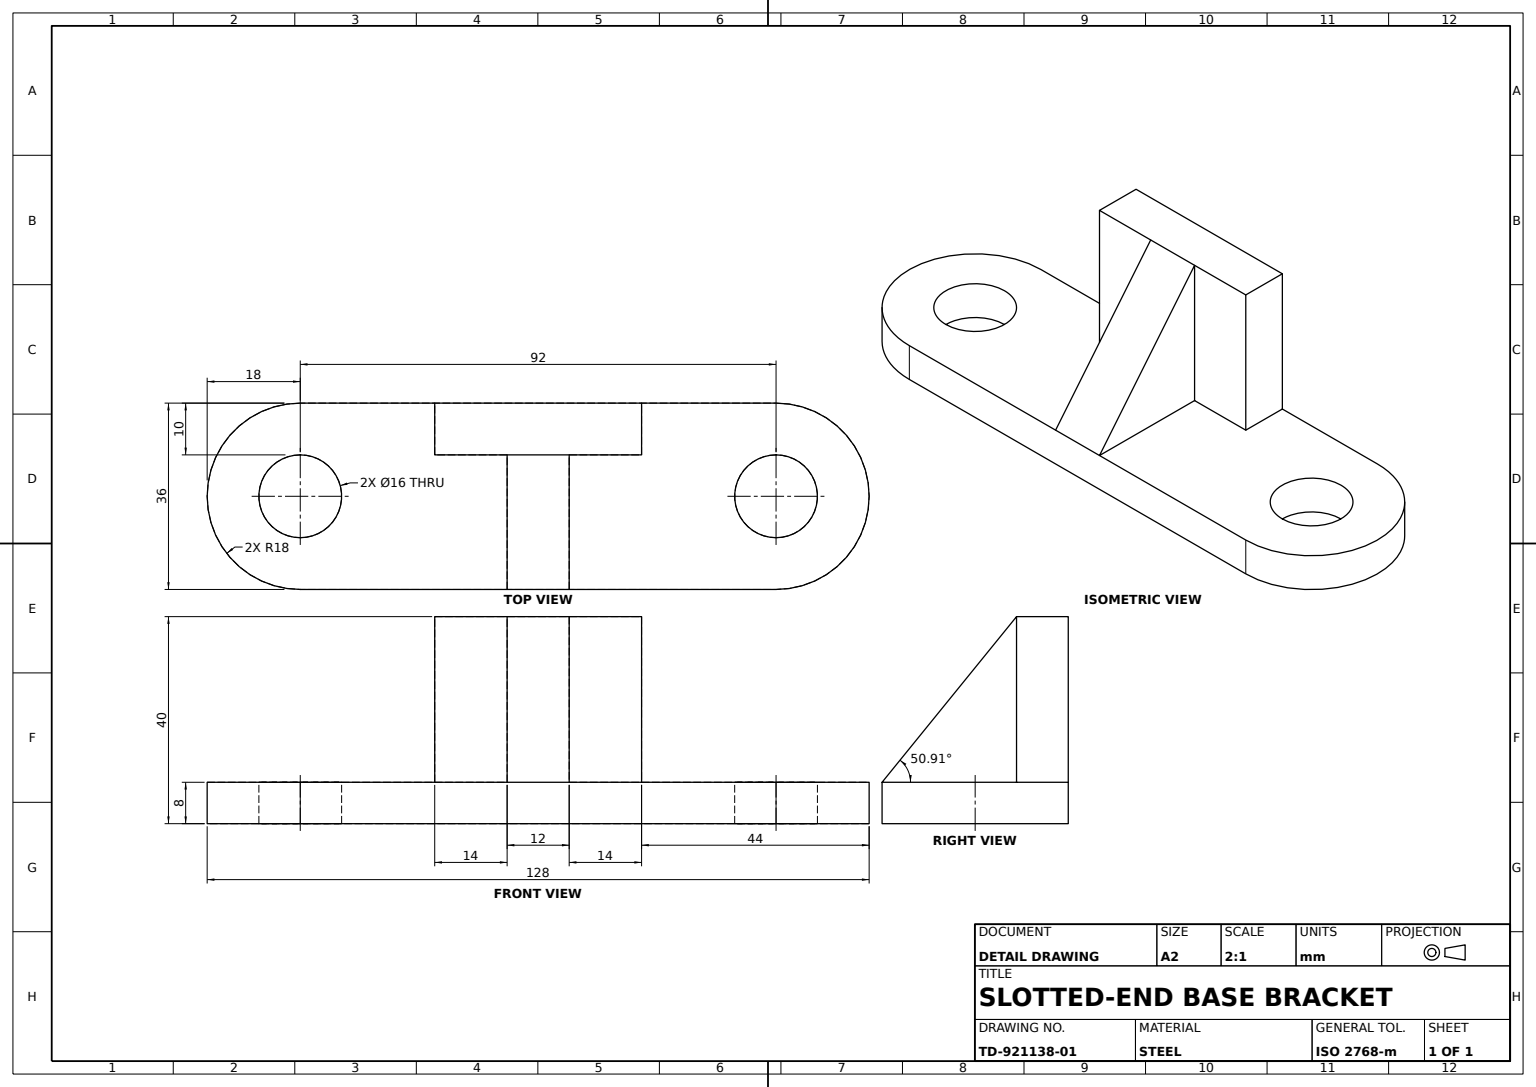
from build123d import *

# Parameters (mm, degrees)
BASE_PLATE_DEPTH          = 8
MOUNTING_HOLES_SKETCH_R   = 8
MOUNTING_HOLES_2X_DEPTH   = 8
UPRIGHT_DEPTH             = 32
SUPPORT_RIB_REACH         = 79.589
SUPPORT_RIB_SKETCH_WALL_W = 198.408374186
SUPPORT_RIB_SKETCH_WALL_H = 12


with BuildPart() as part:
    # Base Plate Sketch → Base Plate (new body)
    with BuildSketch(Plane(origin=(0, 0, 0), x_dir=(1, 0, 0), z_dir=(0, 1, 0))):
        with BuildLine():
            Line((-46, 18), (46, 18))
            ThreePointArc((46, 18), (64, 0), (46, -18))
            Line((46, -18), (-46, -18))
            ThreePointArc((-46, -18), (-64, 0), (-46, 18))
        make_face()
    extrude(amount=BASE_PLATE_DEPTH)

    # Mounting Holes Sketch → Mounting Holes 2x (cut)
    with BuildSketch(Plane(origin=(0, 8, 0), x_dir=(1, 0, 0), z_dir=(0, 1, 0))):
        with Locations(Location((-46, 0, 0), (0, 0, 270))):
            Circle(MOUNTING_HOLES_SKETCH_R)
        with Locations(Location((46, 0, 0), (0, 0, 270))):
            Circle(MOUNTING_HOLES_SKETCH_R)
    extrude(amount=-MOUNTING_HOLES_2X_DEPTH, mode=Mode.SUBTRACT)

    # Upright Sketch → Upright (add)
    with BuildSketch(Plane(origin=(0, 8, 0), x_dir=(1, 0, 0), z_dir=(0, 1, 0))):
        Polygon((0, 18), (-20, 18), (-20, 8), (20, 8), (20, 18), align=None)
    extrude(amount=UPRIGHT_DEPTH)

    # Support Rib Sketch wall → Support Rib (add, up to next)
    with BuildSketch(Plane(origin=(0, 24, 5), x_dir=(0, -0.776114000116, 0.630592625094), z_dir=(0, -0.630592625094, -0.776114000116)), mode=Mode.PRIVATE) as support_rib_sk1:
        Rectangle(SUPPORT_RIB_SKETCH_WALL_W, SUPPORT_RIB_SKETCH_WALL_H)
    support_rib_tool1 = extrude(support_rib_sk1.sketch, amount=SUPPORT_RIB_REACH, mode=Mode.PRIVATE) - part.part
    add(support_rib_tool1.solids().sort_by_distance((0, 24, 5))[0])


solid = part.part
